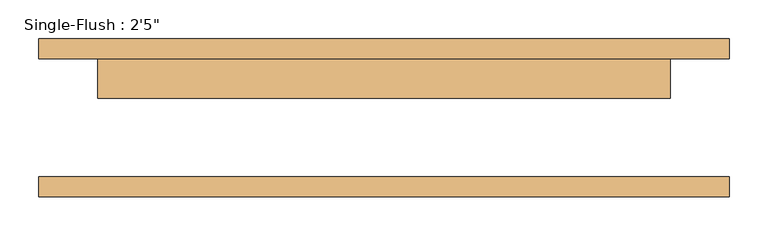
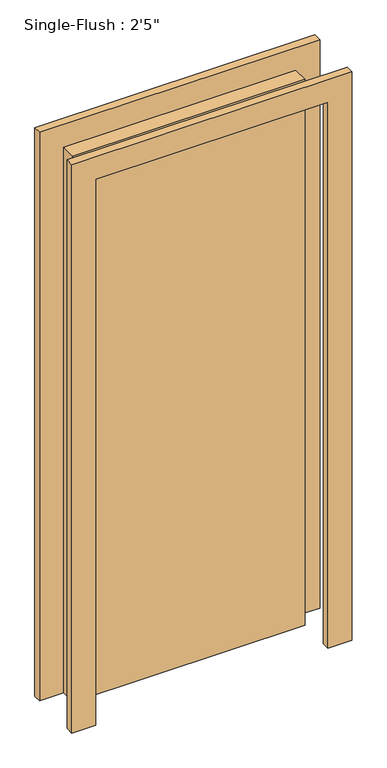
"""IFC4 building model written with IfcOpenShell, lengths in millimetres: door geometry."""

from ifc_helpers import new_model, si_unit, frame, origin, origin_with_axes, place, context, project, spatial, polyline, outline, extrude, source, transform, mapped, element, save


def door_a6948854(model_context):
    return source(origin(), model_context, "Body", "SweptSolid", [
        extrude(outline(polyline([(1905.0, -444.5), (0.0, -444.5), (0.0, -368.3), (1828.8, -368.3), (1828.8, 368.3), (0.0, 368.3), (0.0, 444.5), (1905.0, 444.5), (1905.0, -444.5)])), frame((0.0, 76.2, 0.0), z_axis=(0.0, 1.0, 0.0), x_axis=(0.0, 0.0, 1.0)), (0.0, 0.0, 1.0), 25.4),
        extrude(outline(polyline([(1905.0, 444.5), (1905.0, -444.5), (0.0, -444.5), (0.0, -368.3), (1828.8, -368.3), (1828.8, 368.3), (0.0, 368.3), (0.0, 444.5), (1905.0, 444.5)])), frame((0.0, -101.6, 0.0), z_axis=(0.0, 1.0, 0.0), x_axis=(0.0, 0.0, 1.0)), (0.0, 0.0, 1.0), 25.4),
        extrude(outline(polyline([(368.3, 25.4), (-368.3, 25.4), (-368.3, 76.2), (368.3, 76.2), (368.3, 25.4)])), origin_with_axes(), (0.0, 0.0, 1.0), 1828.8),
    ])


if __name__ == "__main__":
    model = new_model("IFC4")
    model_context = context("Model", 3, world=origin())
    ifc_project = project(units=[si_unit("LENGTHUNIT", "METRE", prefix="MILLI")], contexts=[model_context])
    site = spatial("IfcSite", under=ifc_project)
    building = spatial("IfcBuilding", under=site)
    placement = place(None, origin())
    door_shape = door_a6948854(model_context)
    element("IfcDoor", 1, ObjectType="Single-Flush : 2'5\"", at=placement, inside=building, context=model_context, shape_type="MappedRepresentation", body=[
        mapped(door_shape, transform((0.0, 0.0, 0.0), x_axis=(1.0, 0.0, 0.0), y_axis=(0.0, 1.0, 0.0), z_axis=(0.0, 0.0, 1.0))),
    ])
    save(model, "model.ifc")

# Revit data of these elements
# Type "Single-Flush : 2'5\""
#   Type Mark = "8"
#   Construction Type Id = "MDOOR"
#   Assembly Code = "C1020"
#   Analytic Construction = "Metal"
#   Thickness = 0' - 2"
#   Heat Transfer Coefficient (U) = 0.651978 BTU/(h·ft²·°F)
#   Height = 6' - 0"
#   Trim Projection Ext = 0' - 1"
#   Trim Projection Int = 0' - 1"
#   Trim Width = 0' - 3"
#   Width = 2' - 5"
#   Define Thermal Properties by = 1
#   Door Material = Door - Panel
#   Frame Material = Door - Frame
#   Visual Light Transmittance = 0
#   Solar Heat Gain Coefficient = 0
#   Function = (empty or 0)
#   Wall Closure = (empty or 0)
# Element 1 (IfcDoor, "Single-Flush : 2'5\"")
#   Materials on its faces: "Door - Frame", "Door - Panel"
# Materials
#   "Door - Panel": class "Wood", colour RGB 210 159 95, transparency 0, Cost = 0
#   "Door - Frame": colour RGB 118 70 51, transparency 0, Cost = 0
